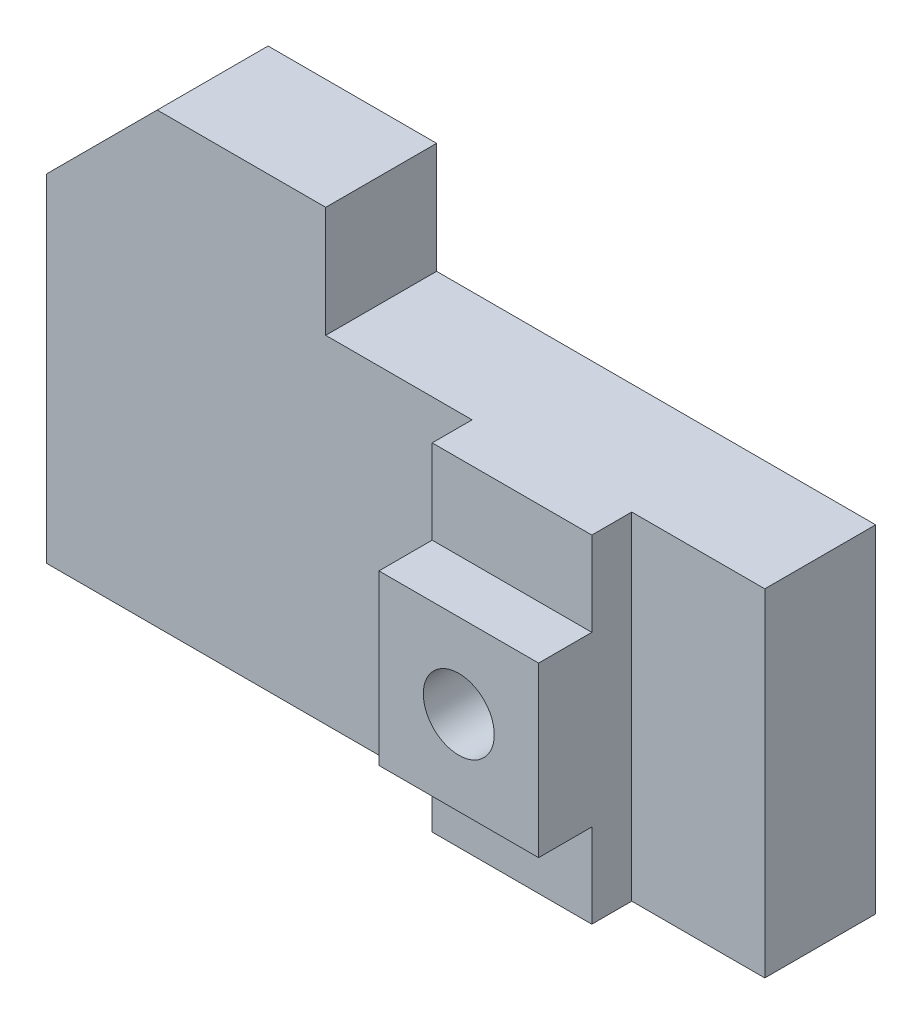
ISO-10303-21;
HEADER;
FILE_DESCRIPTION(('STEP AP214'),'2;1');
FILE_NAME('part.step','',(''),(''),'','','');
FILE_SCHEMA(('AUTOMOTIVE_DESIGN { 1 0 10303 214 1 1 1 1 }'));
ENDSEC;
DATA;
#1=APPLICATION_CONTEXT('core data for automotive mechanical design processes');
#2=APPLICATION_PROTOCOL_DEFINITION('international standard','automotive_design',2000,#1);
#3=PRODUCT_CONTEXT('',#1,'mechanical');
#4=PRODUCT('Part','Part','',(#3));
#5=PRODUCT_RELATED_PRODUCT_CATEGORY('part','',(#4));
#6=PRODUCT_DEFINITION_FORMATION('','',#4);
#7=PRODUCT_DEFINITION_CONTEXT('part definition',#1,'design');
#8=PRODUCT_DEFINITION('design','',#6,#7);
#9=PRODUCT_DEFINITION_SHAPE('','',#8);
#10=(LENGTH_UNIT() NAMED_UNIT(*) SI_UNIT(.MILLI.,.METRE.));
#11=(NAMED_UNIT(*) PLANE_ANGLE_UNIT() SI_UNIT($,.RADIAN.));
#12=(NAMED_UNIT(*) SI_UNIT($,.STERADIAN.) SOLID_ANGLE_UNIT());
#13=UNCERTAINTY_MEASURE_WITH_UNIT(LENGTH_MEASURE(1.E-05),#10,'distance_accuracy_value','');
#14=(GEOMETRIC_REPRESENTATION_CONTEXT(3) GLOBAL_UNCERTAINTY_ASSIGNED_CONTEXT((#13)) GLOBAL_UNIT_ASSIGNED_CONTEXT((#10,
#11,#12)) REPRESENTATION_CONTEXT('',''));
#15=CARTESIAN_POINT('',(0.,0.,0.));
#16=DIRECTION('',(0.,0.,1.));
#17=DIRECTION('',(1.,0.,0.));
#18=AXIS2_PLACEMENT_3D('',#15,#16,#17);
#19=CARTESIAN_POINT('',(0.,0.,34.));
#20=DIRECTION('',(0.,0.,-1.));
#21=DIRECTION('',(-1.,0.,0.));
#22=AXIS2_PLACEMENT_3D('',#19,#20,#21);
#23=PLANE('',#22);
#24=DIRECTION('',(-1.,0.,0.));
#25=VECTOR('',#24,1.);
#26=CARTESIAN_POINT('',(96.,57.,34.));
#27=LINE('',#26,#25);
#28=CARTESIAN_POINT('',(132.,57.,34.));
#29=VERTEX_POINT('',#28);
#30=CARTESIAN_POINT('',(96.,57.,34.));
#31=VERTEX_POINT('',#30);
#32=EDGE_CURVE('E173',#29,#31,#27,.T.);
#33=ORIENTED_EDGE('',*,*,#32,.F.);
#34=DIRECTION('',(0.,1.,0.));
#35=VECTOR('',#34,1.);
#36=CARTESIAN_POINT('',(132.,76.,34.));
#37=LINE('',#36,#35);
#38=CARTESIAN_POINT('',(132.,76.,34.));
#39=VERTEX_POINT('',#38);
#40=EDGE_CURVE('E187',#29,#39,#37,.T.);
#41=ORIENTED_EDGE('',*,*,#40,.T.);
#42=DIRECTION('',(-1.,0.,0.));
#43=VECTOR('',#42,1.);
#44=CARTESIAN_POINT('',(96.,76.,34.));
#45=LINE('',#44,#43);
#46=CARTESIAN_POINT('',(96.,76.,34.));
#47=VERTEX_POINT('',#46);
#48=EDGE_CURVE('E195',#39,#47,#45,.T.);
#49=ORIENTED_EDGE('',*,*,#48,.T.);
#50=DIRECTION('',(0.,-1.,0.));
#51=VECTOR('',#50,1.);
#52=CARTESIAN_POINT('',(96.,0.,34.));
#53=LINE('',#52,#51);
#54=EDGE_CURVE('E68',#47,#31,#53,.T.);
#55=ORIENTED_EDGE('',*,*,#54,.T.);
#56=EDGE_LOOP('',(#33,#41,#49,#55));
#57=FACE_BOUND('',#56,.T.);
#58=ADVANCED_FACE('F44',(#57),#23,.F.);
#59=DIRECTION('',(1.,0.,0.));
#60=VECTOR('',#59,1.);
#61=CARTESIAN_POINT('',(132.,19.,34.));
#62=LINE('',#61,#60);
#63=CARTESIAN_POINT('',(96.,19.,34.));
#64=VERTEX_POINT('',#63);
#65=CARTESIAN_POINT('',(132.,19.,34.));
#66=VERTEX_POINT('',#65);
#67=EDGE_CURVE('E58',#64,#66,#62,.T.);
#68=ORIENTED_EDGE('',*,*,#67,.F.);
#69=CARTESIAN_POINT('',(96.,0.,34.));
#70=VERTEX_POINT('',#69);
#71=EDGE_CURVE('E176',#64,#70,#53,.T.);
#72=ORIENTED_EDGE('',*,*,#71,.T.);
#73=DIRECTION('',(1.,0.,0.));
#74=VECTOR('',#73,1.);
#75=CARTESIAN_POINT('',(132.,0.,34.));
#76=LINE('',#75,#74);
#77=CARTESIAN_POINT('',(132.,0.,34.));
#78=VERTEX_POINT('',#77);
#79=EDGE_CURVE('E188',#70,#78,#76,.T.);
#80=ORIENTED_EDGE('',*,*,#79,.T.);
#81=EDGE_CURVE('E189',#78,#66,#37,.T.);
#82=ORIENTED_EDGE('',*,*,#81,.T.);
#83=EDGE_LOOP('',(#68,#72,#80,#82));
#84=FACE_BOUND('',#83,.T.);
#85=ADVANCED_FACE('F286',(#84),#23,.F.);
#86=CARTESIAN_POINT('',(0.,0.,25.));
#87=DIRECTION('',(0.,0.,-1.));
#88=DIRECTION('',(-1.,0.,0.));
#89=AXIS2_PLACEMENT_3D('',#86,#87,#88);
#90=PLANE('',#89);
#91=DIRECTION('',(0.,-1.,0.));
#92=VECTOR('',#91,1.);
#93=CARTESIAN_POINT('',(96.,0.,25.));
#94=LINE('',#93,#92);
#95=CARTESIAN_POINT('',(96.,76.,25.));
#96=VERTEX_POINT('',#95);
#97=CARTESIAN_POINT('',(96.,0.,25.));
#98=VERTEX_POINT('',#97);
#99=EDGE_CURVE('E179',#96,#98,#94,.T.);
#100=ORIENTED_EDGE('',*,*,#99,.F.);
#101=DIRECTION('',(-1.,0.,0.));
#102=VECTOR('',#101,1.);
#103=CARTESIAN_POINT('',(162.,76.,25.));
#104=LINE('',#103,#102);
#105=CARTESIAN_POINT('',(63.,76.,25.));
#106=VERTEX_POINT('',#105);
#107=EDGE_CURVE('E245',#96,#106,#104,.T.);
#108=ORIENTED_EDGE('',*,*,#107,.T.);
#109=DIRECTION('',(0.,1.,0.));
#110=VECTOR('',#109,1.);
#111=CARTESIAN_POINT('',(63.,76.,25.));
#112=LINE('',#111,#110);
#113=CARTESIAN_POINT('',(63.,101.,25.));
#114=VERTEX_POINT('',#113);
#115=EDGE_CURVE('E208',#106,#114,#112,.T.);
#116=ORIENTED_EDGE('',*,*,#115,.T.);
#117=DIRECTION('',(-1.,0.,0.));
#118=VECTOR('',#117,1.);
#119=CARTESIAN_POINT('',(63.,101.,25.));
#120=LINE('',#119,#118);
#121=CARTESIAN_POINT('',(25.,101.,25.));
#122=VERTEX_POINT('',#121);
#123=EDGE_CURVE('E222',#114,#122,#120,.T.);
#124=ORIENTED_EDGE('',*,*,#123,.T.);
#125=DIRECTION('',(-0.707106781186547,-0.707106781186548,0.));
#126=VECTOR('',#125,1.);
#127=CARTESIAN_POINT('',(25.,101.,25.));
#128=LINE('',#127,#126);
#129=CARTESIAN_POINT('',(0.,76.,25.));
#130=VERTEX_POINT('',#129);
#131=EDGE_CURVE('E213',#122,#130,#128,.T.);
#132=ORIENTED_EDGE('',*,*,#131,.T.);
#133=DIRECTION('',(0.,-1.,0.));
#134=VECTOR('',#133,1.);
#135=CARTESIAN_POINT('',(0.,0.,25.));
#136=LINE('',#135,#134);
#137=CARTESIAN_POINT('',(0.,0.,25.));
#138=VERTEX_POINT('',#137);
#139=EDGE_CURVE('E233',#130,#138,#136,.T.);
#140=ORIENTED_EDGE('',*,*,#139,.T.);
#141=DIRECTION('',(1.,0.,0.));
#142=VECTOR('',#141,1.);
#143=CARTESIAN_POINT('',(0.,0.,25.));
#144=LINE('',#143,#142);
#145=EDGE_CURVE('E236',#138,#98,#144,.T.);
#146=ORIENTED_EDGE('',*,*,#145,.T.);
#147=EDGE_LOOP('',(#100,#108,#116,#124,#132,#140,#146));
#148=FACE_BOUND('',#147,.T.);
#149=ADVANCED_FACE('F287',(#148),#90,.F.);
#150=DIRECTION('',(0.,1.,0.));
#151=VECTOR('',#150,1.);
#152=CARTESIAN_POINT('',(132.,76.,25.));
#153=LINE('',#152,#151);
#154=CARTESIAN_POINT('',(132.,0.,25.));
#155=VERTEX_POINT('',#154);
#156=CARTESIAN_POINT('',(132.,76.,25.));
#157=VERTEX_POINT('',#156);
#158=EDGE_CURVE('E180',#155,#157,#153,.T.);
#159=ORIENTED_EDGE('',*,*,#158,.F.);
#160=CARTESIAN_POINT('',(162.,0.,25.));
#161=VERTEX_POINT('',#160);
#162=EDGE_CURVE('E237',#155,#161,#144,.T.);
#163=ORIENTED_EDGE('',*,*,#162,.T.);
#164=DIRECTION('',(0.,1.,0.));
#165=VECTOR('',#164,1.);
#166=CARTESIAN_POINT('',(162.,0.,25.));
#167=LINE('',#166,#165);
#168=CARTESIAN_POINT('',(162.,76.,25.));
#169=VERTEX_POINT('',#168);
#170=EDGE_CURVE('E238',#161,#169,#167,.T.);
#171=ORIENTED_EDGE('',*,*,#170,.T.);
#172=EDGE_CURVE('E241',#169,#157,#104,.T.);
#173=ORIENTED_EDGE('',*,*,#172,.T.);
#174=EDGE_LOOP('',(#159,#163,#171,#173));
#175=FACE_BOUND('',#174,.T.);
#176=ADVANCED_FACE('F278',(#175),#90,.F.);
#177=CARTESIAN_POINT('',(0.,0.,25.));
#178=DIRECTION('',(0.,1.,0.));
#179=DIRECTION('',(0.,0.,1.));
#180=AXIS2_PLACEMENT_3D('',#177,#178,#179);
#181=PLANE('',#180);
#182=DIRECTION('',(1.,0.,0.));
#183=VECTOR('',#182,1.);
#184=CARTESIAN_POINT('',(0.,0.,0.));
#185=LINE('',#184,#183);
#186=CARTESIAN_POINT('',(0.,0.,0.));
#187=VERTEX_POINT('',#186);
#188=CARTESIAN_POINT('',(162.,0.,0.));
#189=VERTEX_POINT('',#188);
#190=EDGE_CURVE('E226',#187,#189,#185,.T.);
#191=ORIENTED_EDGE('',*,*,#190,.T.);
#192=DIRECTION('',(0.,0.,-1.));
#193=VECTOR('',#192,1.);
#194=CARTESIAN_POINT('',(162.,0.,25.));
#195=LINE('',#194,#193);
#196=EDGE_CURVE('E52',#161,#189,#195,.T.);
#197=ORIENTED_EDGE('',*,*,#196,.F.);
#198=ORIENTED_EDGE('',*,*,#162,.F.);
#199=DIRECTION('',(0.,0.,-1.));
#200=VECTOR('',#199,1.);
#201=CARTESIAN_POINT('',(132.,0.,34.));
#202=LINE('',#201,#200);
#203=EDGE_CURVE('E202',#78,#155,#202,.T.);
#204=ORIENTED_EDGE('',*,*,#203,.F.);
#205=ORIENTED_EDGE('',*,*,#79,.F.);
#206=DIRECTION('',(0.,0.,-1.));
#207=VECTOR('',#206,1.);
#208=CARTESIAN_POINT('',(96.,0.,34.));
#209=LINE('',#208,#207);
#210=EDGE_CURVE('E192',#70,#98,#209,.T.);
#211=ORIENTED_EDGE('',*,*,#210,.T.);
#212=ORIENTED_EDGE('',*,*,#145,.F.);
#213=DIRECTION('',(0.,0.,-1.));
#214=VECTOR('',#213,1.);
#215=CARTESIAN_POINT('',(0.,0.,25.));
#216=LINE('',#215,#214);
#217=EDGE_CURVE('E11',#138,#187,#216,.T.);
#218=ORIENTED_EDGE('',*,*,#217,.T.);
#219=EDGE_LOOP('',(#191,#197,#198,#204,#205,#211,#212,#218));
#220=FACE_BOUND('',#219,.T.);
#221=ADVANCED_FACE('F50',(#220),#181,.F.);
#222=CARTESIAN_POINT('',(162.,0.,25.));
#223=DIRECTION('',(-1.,0.,0.));
#224=DIRECTION('',(0.,0.,1.));
#225=AXIS2_PLACEMENT_3D('',#222,#223,#224);
#226=PLANE('',#225);
#227=DIRECTION('',(0.,1.,0.));
#228=VECTOR('',#227,1.);
#229=CARTESIAN_POINT('',(162.,0.,0.));
#230=LINE('',#229,#228);
#231=CARTESIAN_POINT('',(162.,76.,0.));
#232=VERTEX_POINT('',#231);
#233=EDGE_CURVE('E250',#189,#232,#230,.T.);
#234=ORIENTED_EDGE('',*,*,#233,.T.);
#235=DIRECTION('',(0.,0.,-1.));
#236=VECTOR('',#235,1.);
#237=CARTESIAN_POINT('',(162.,76.,25.));
#238=LINE('',#237,#236);
#239=EDGE_CURVE('E258',#169,#232,#238,.T.);
#240=ORIENTED_EDGE('',*,*,#239,.F.);
#241=ORIENTED_EDGE('',*,*,#170,.F.);
#242=ORIENTED_EDGE('',*,*,#196,.T.);
#243=EDGE_LOOP('',(#234,#240,#241,#242));
#244=FACE_BOUND('',#243,.T.);
#245=ADVANCED_FACE('F263',(#244),#226,.F.);
#246=CARTESIAN_POINT('',(0.,76.,25.));
#247=DIRECTION('',(0.,-1.,0.));
#248=DIRECTION('',(0.,0.,-1.));
#249=AXIS2_PLACEMENT_3D('',#246,#247,#248);
#250=PLANE('',#249);
#251=DIRECTION('',(-1.,0.,0.));
#252=VECTOR('',#251,1.);
#253=CARTESIAN_POINT('',(0.,76.,0.));
#254=LINE('',#253,#252);
#255=CARTESIAN_POINT('',(63.,76.,0.));
#256=VERTEX_POINT('',#255);
#257=EDGE_CURVE('E249',#232,#256,#254,.T.);
#258=ORIENTED_EDGE('',*,*,#257,.T.);
#259=DIRECTION('',(0.,0.,1.));
#260=VECTOR('',#259,1.);
#261=CARTESIAN_POINT('',(63.,76.,0.));
#262=LINE('',#261,#260);
#263=EDGE_CURVE('E217',#256,#106,#262,.T.);
#264=ORIENTED_EDGE('',*,*,#263,.T.);
#265=ORIENTED_EDGE('',*,*,#107,.F.);
#266=DIRECTION('',(0.,0.,-1.));
#267=VECTOR('',#266,1.);
#268=CARTESIAN_POINT('',(96.,76.,34.));
#269=LINE('',#268,#267);
#270=EDGE_CURVE('E200',#47,#96,#269,.T.);
#271=ORIENTED_EDGE('',*,*,#270,.F.);
#272=ORIENTED_EDGE('',*,*,#48,.F.);
#273=DIRECTION('',(0.,0.,-1.));
#274=VECTOR('',#273,1.);
#275=CARTESIAN_POINT('',(132.,76.,34.));
#276=LINE('',#275,#274);
#277=EDGE_CURVE('E205',#39,#157,#276,.T.);
#278=ORIENTED_EDGE('',*,*,#277,.T.);
#279=ORIENTED_EDGE('',*,*,#172,.F.);
#280=ORIENTED_EDGE('',*,*,#239,.T.);
#281=EDGE_LOOP('',(#258,#264,#265,#271,#272,#278,#279,#280));
#282=FACE_BOUND('',#281,.T.);
#283=ADVANCED_FACE('F273',(#282),#250,.F.);
#284=CARTESIAN_POINT('',(0.,51.,25.));
#285=DIRECTION('',(1.,0.,0.));
#286=DIRECTION('',(0.,0.,-1.));
#287=AXIS2_PLACEMENT_3D('',#284,#285,#286);
#288=PLANE('',#287);
#289=DIRECTION('',(0.,-1.,0.));
#290=VECTOR('',#289,1.);
#291=CARTESIAN_POINT('',(0.,51.,0.));
#292=LINE('',#291,#290);
#293=CARTESIAN_POINT('',(0.,76.,0.));
#294=VERTEX_POINT('',#293);
#295=EDGE_CURVE('E240',#294,#187,#292,.T.);
#296=ORIENTED_EDGE('',*,*,#295,.T.);
#297=ORIENTED_EDGE('',*,*,#217,.F.);
#298=ORIENTED_EDGE('',*,*,#139,.F.);
#299=DIRECTION('',(0.,0.,-1.));
#300=VECTOR('',#299,1.);
#301=CARTESIAN_POINT('',(0.,76.,25.));
#302=LINE('',#301,#300);
#303=EDGE_CURVE('E244',#130,#294,#302,.T.);
#304=ORIENTED_EDGE('',*,*,#303,.T.);
#305=EDGE_LOOP('',(#296,#297,#298,#304));
#306=FACE_BOUND('',#305,.T.);
#307=ADVANCED_FACE('F349',(#306),#288,.F.);
#308=CARTESIAN_POINT('',(0.,0.,0.));
#309=DIRECTION('',(0.,0.,-1.));
#310=DIRECTION('',(-1.,0.,0.));
#311=AXIS2_PLACEMENT_3D('',#308,#309,#310);
#312=PLANE('',#311);
#313=ORIENTED_EDGE('',*,*,#190,.F.);
#314=ORIENTED_EDGE('',*,*,#295,.F.);
#315=DIRECTION('',(-0.707106781186547,-0.707106781186548,0.));
#316=VECTOR('',#315,1.);
#317=CARTESIAN_POINT('',(25.,101.,0.));
#318=LINE('',#317,#316);
#319=CARTESIAN_POINT('',(25.,101.,0.));
#320=VERTEX_POINT('',#319);
#321=EDGE_CURVE('E216',#320,#294,#318,.T.);
#322=ORIENTED_EDGE('',*,*,#321,.F.);
#323=DIRECTION('',(-1.,0.,0.));
#324=VECTOR('',#323,1.);
#325=CARTESIAN_POINT('',(63.,101.,0.));
#326=LINE('',#325,#324);
#327=CARTESIAN_POINT('',(63.,101.,0.));
#328=VERTEX_POINT('',#327);
#329=EDGE_CURVE('E215',#328,#320,#326,.T.);
#330=ORIENTED_EDGE('',*,*,#329,.F.);
#331=DIRECTION('',(0.,1.,0.));
#332=VECTOR('',#331,1.);
#333=CARTESIAN_POINT('',(63.,76.,0.));
#334=LINE('',#333,#332);
#335=EDGE_CURVE('E207',#256,#328,#334,.T.);
#336=ORIENTED_EDGE('',*,*,#335,.F.);
#337=ORIENTED_EDGE('',*,*,#257,.F.);
#338=ORIENTED_EDGE('',*,*,#233,.F.);
#339=EDGE_LOOP('',(#313,#314,#322,#330,#336,#337,#338));
#340=FACE_BOUND('',#339,.T.);
#341=ADVANCED_FACE('F267',(#340),#312,.T.);
#342=CARTESIAN_POINT('',(25.,101.,0.));
#343=DIRECTION('',(-0.707106781186548,0.707106781186547,0.));
#344=DIRECTION('',(-0.707106781186547,-0.707106781186548,0.));
#345=AXIS2_PLACEMENT_3D('',#342,#343,#344);
#346=PLANE('',#345);
#347=ORIENTED_EDGE('',*,*,#131,.F.);
#348=DIRECTION('',(0.,0.,1.));
#349=VECTOR('',#348,1.);
#350=CARTESIAN_POINT('',(25.,101.,0.));
#351=LINE('',#350,#349);
#352=EDGE_CURVE('E228',#320,#122,#351,.T.);
#353=ORIENTED_EDGE('',*,*,#352,.F.);
#354=ORIENTED_EDGE('',*,*,#321,.T.);
#355=ORIENTED_EDGE('',*,*,#303,.F.);
#356=EDGE_LOOP('',(#347,#353,#354,#355));
#357=FACE_BOUND('',#356,.T.);
#358=ADVANCED_FACE('F331',(#357),#346,.T.);
#359=CARTESIAN_POINT('',(63.,101.,0.));
#360=DIRECTION('',(0.,1.,0.));
#361=DIRECTION('',(0.,0.,1.));
#362=AXIS2_PLACEMENT_3D('',#359,#360,#361);
#363=PLANE('',#362);
#364=ORIENTED_EDGE('',*,*,#123,.F.);
#365=DIRECTION('',(0.,0.,1.));
#366=VECTOR('',#365,1.);
#367=CARTESIAN_POINT('',(63.,101.,0.));
#368=LINE('',#367,#366);
#369=EDGE_CURVE('E227',#328,#114,#368,.T.);
#370=ORIENTED_EDGE('',*,*,#369,.F.);
#371=ORIENTED_EDGE('',*,*,#329,.T.);
#372=ORIENTED_EDGE('',*,*,#352,.T.);
#373=EDGE_LOOP('',(#364,#370,#371,#372));
#374=FACE_BOUND('',#373,.T.);
#375=ADVANCED_FACE('F340',(#374),#363,.T.);
#376=CARTESIAN_POINT('',(63.,76.,0.));
#377=DIRECTION('',(1.,0.,0.));
#378=DIRECTION('',(0.,0.,-1.));
#379=AXIS2_PLACEMENT_3D('',#376,#377,#378);
#380=PLANE('',#379);
#381=ORIENTED_EDGE('',*,*,#115,.F.);
#382=ORIENTED_EDGE('',*,*,#263,.F.);
#383=ORIENTED_EDGE('',*,*,#335,.T.);
#384=ORIENTED_EDGE('',*,*,#369,.T.);
#385=EDGE_LOOP('',(#381,#382,#383,#384));
#386=FACE_BOUND('',#385,.T.);
#387=ADVANCED_FACE('F334',(#386),#380,.T.);
#388=CARTESIAN_POINT('',(132.,76.,34.));
#389=DIRECTION('',(-1.,0.,0.));
#390=DIRECTION('',(0.,0.,1.));
#391=AXIS2_PLACEMENT_3D('',#388,#389,#390);
#392=PLANE('',#391);
#393=ORIENTED_EDGE('',*,*,#158,.T.);
#394=ORIENTED_EDGE('',*,*,#277,.F.);
#395=ORIENTED_EDGE('',*,*,#40,.F.);
#396=DIRECTION('',(0.,0.,-1.));
#397=VECTOR('',#396,1.);
#398=CARTESIAN_POINT('',(132.,57.,46.));
#399=LINE('',#398,#397);
#400=CARTESIAN_POINT('',(132.,57.,46.));
#401=VERTEX_POINT('',#400);
#402=EDGE_CURVE('E185',#401,#29,#399,.T.);
#403=ORIENTED_EDGE('',*,*,#402,.F.);
#404=DIRECTION('',(0.,1.,0.));
#405=VECTOR('',#404,1.);
#406=CARTESIAN_POINT('',(132.,57.,46.));
#407=LINE('',#406,#405);
#408=CARTESIAN_POINT('',(132.,19.,46.));
#409=VERTEX_POINT('',#408);
#410=EDGE_CURVE('E161',#409,#401,#407,.T.);
#411=ORIENTED_EDGE('',*,*,#410,.F.);
#412=DIRECTION('',(0.,0.,-1.));
#413=VECTOR('',#412,1.);
#414=CARTESIAN_POINT('',(132.,19.,46.));
#415=LINE('',#414,#413);
#416=EDGE_CURVE('E158',#409,#66,#415,.T.);
#417=ORIENTED_EDGE('',*,*,#416,.T.);
#418=ORIENTED_EDGE('',*,*,#81,.F.);
#419=ORIENTED_EDGE('',*,*,#203,.T.);
#420=EDGE_LOOP('',(#393,#394,#395,#403,#411,#417,#418,#419));
#421=FACE_BOUND('',#420,.T.);
#422=ADVANCED_FACE('F285',(#421),#392,.F.);
#423=CARTESIAN_POINT('',(96.,0.,34.));
#424=DIRECTION('',(1.,0.,0.));
#425=DIRECTION('',(0.,0.,-1.));
#426=AXIS2_PLACEMENT_3D('',#423,#424,#425);
#427=PLANE('',#426);
#428=ORIENTED_EDGE('',*,*,#99,.T.);
#429=ORIENTED_EDGE('',*,*,#210,.F.);
#430=ORIENTED_EDGE('',*,*,#71,.F.);
#431=DIRECTION('',(0.,0.,-1.));
#432=VECTOR('',#431,1.);
#433=CARTESIAN_POINT('',(96.,19.,46.));
#434=LINE('',#433,#432);
#435=CARTESIAN_POINT('',(96.,19.,46.));
#436=VERTEX_POINT('',#435);
#437=EDGE_CURVE('E156',#436,#64,#434,.T.);
#438=ORIENTED_EDGE('',*,*,#437,.F.);
#439=DIRECTION('',(0.,-1.,0.));
#440=VECTOR('',#439,1.);
#441=CARTESIAN_POINT('',(96.,19.,46.));
#442=LINE('',#441,#440);
#443=CARTESIAN_POINT('',(96.,57.,46.));
#444=VERTEX_POINT('',#443);
#445=EDGE_CURVE('E165',#444,#436,#442,.T.);
#446=ORIENTED_EDGE('',*,*,#445,.F.);
#447=DIRECTION('',(0.,0.,-1.));
#448=VECTOR('',#447,1.);
#449=CARTESIAN_POINT('',(96.,57.,46.));
#450=LINE('',#449,#448);
#451=EDGE_CURVE('E292',#444,#31,#450,.T.);
#452=ORIENTED_EDGE('',*,*,#451,.T.);
#453=ORIENTED_EDGE('',*,*,#54,.F.);
#454=ORIENTED_EDGE('',*,*,#270,.T.);
#455=EDGE_LOOP('',(#428,#429,#430,#438,#446,#452,#453,#454));
#456=FACE_BOUND('',#455,.T.);
#457=ADVANCED_FACE('F172',(#456),#427,.F.);
#458=CARTESIAN_POINT('',(132.,19.,46.));
#459=DIRECTION('',(0.,1.,0.));
#460=DIRECTION('',(0.,0.,1.));
#461=AXIS2_PLACEMENT_3D('',#458,#459,#460);
#462=PLANE('',#461);
#463=ORIENTED_EDGE('',*,*,#67,.T.);
#464=ORIENTED_EDGE('',*,*,#416,.F.);
#465=DIRECTION('',(1.,0.,0.));
#466=VECTOR('',#465,1.);
#467=CARTESIAN_POINT('',(132.,19.,46.));
#468=LINE('',#467,#466);
#469=EDGE_CURVE('E155',#436,#409,#468,.T.);
#470=ORIENTED_EDGE('',*,*,#469,.F.);
#471=ORIENTED_EDGE('',*,*,#437,.T.);
#472=EDGE_LOOP('',(#463,#464,#470,#471));
#473=FACE_BOUND('',#472,.T.);
#474=ADVANCED_FACE('F152',(#473),#462,.F.);
#475=CARTESIAN_POINT('',(96.,57.,46.));
#476=DIRECTION('',(0.,-1.,0.));
#477=DIRECTION('',(0.,0.,-1.));
#478=AXIS2_PLACEMENT_3D('',#475,#476,#477);
#479=PLANE('',#478);
#480=ORIENTED_EDGE('',*,*,#32,.T.);
#481=ORIENTED_EDGE('',*,*,#451,.F.);
#482=DIRECTION('',(-1.,0.,0.));
#483=VECTOR('',#482,1.);
#484=CARTESIAN_POINT('',(96.,57.,46.));
#485=LINE('',#484,#483);
#486=EDGE_CURVE('E170',#401,#444,#485,.T.);
#487=ORIENTED_EDGE('',*,*,#486,.F.);
#488=ORIENTED_EDGE('',*,*,#402,.T.);
#489=EDGE_LOOP('',(#480,#481,#487,#488));
#490=FACE_BOUND('',#489,.T.);
#491=ADVANCED_FACE('F316',(#490),#479,.F.);
#492=CARTESIAN_POINT('',(0.,0.,46.));
#493=DIRECTION('',(0.,0.,-1.));
#494=DIRECTION('',(-1.,0.,0.));
#495=AXIS2_PLACEMENT_3D('',#492,#493,#494);
#496=PLANE('',#495);
#497=CARTESIAN_POINT('',(114.,38.,46.));
#498=DIRECTION('',(0.,0.,1.));
#499=DIRECTION('',(1.,0.,0.));
#500=AXIS2_PLACEMENT_3D('',#497,#498,#499);
#501=CIRCLE('',#500,8.);
#502=CARTESIAN_POINT('',(122.,38.,46.));
#503=VERTEX_POINT('',#502);
#504=EDGE_CURVE('E301',#503,#503,#501,.T.);
#505=ORIENTED_EDGE('',*,*,#504,.F.);
#506=EDGE_LOOP('',(#505));
#507=FACE_BOUND('',#506,.T.);
#508=ORIENTED_EDGE('',*,*,#445,.T.);
#509=ORIENTED_EDGE('',*,*,#469,.T.);
#510=ORIENTED_EDGE('',*,*,#410,.T.);
#511=ORIENTED_EDGE('',*,*,#486,.T.);
#512=EDGE_LOOP('',(#508,#509,#510,#511));
#513=FACE_BOUND('',#512,.T.);
#514=ADVANCED_FACE('F164',(#507,#513),#496,.F.);
#515=CARTESIAN_POINT('',(114.,38.,26.));
#516=DIRECTION('',(0.,0.,1.));
#517=DIRECTION('',(1.,0.,0.));
#518=AXIS2_PLACEMENT_3D('',#515,#516,#517);
#519=CYLINDRICAL_SURFACE('',#518,8.);
#520=CARTESIAN_POINT('',(114.,38.,26.));
#521=DIRECTION('',(0.,0.,1.));
#522=DIRECTION('',(1.,0.,0.));
#523=AXIS2_PLACEMENT_3D('',#520,#521,#522);
#524=CIRCLE('',#523,8.);
#525=CARTESIAN_POINT('',(122.,38.,26.));
#526=VERTEX_POINT('',#525);
#527=EDGE_CURVE('E296',#526,#526,#524,.T.);
#528=ORIENTED_EDGE('',*,*,#527,.F.);
#529=EDGE_LOOP('',(#528));
#530=FACE_BOUND('',#529,.T.);
#531=ORIENTED_EDGE('',*,*,#504,.T.);
#532=EDGE_LOOP('',(#531));
#533=FACE_BOUND('',#532,.T.);
#534=ADVANCED_FACE('F310',(#530,#533),#519,.F.);
#535=CARTESIAN_POINT('',(114.,38.,26.));
#536=DIRECTION('',(0.,0.,1.));
#537=DIRECTION('',(1.,0.,0.));
#538=AXIS2_PLACEMENT_3D('',#535,#536,#537);
#539=PLANE('',#538);
#540=ORIENTED_EDGE('',*,*,#527,.T.);
#541=EDGE_LOOP('',(#540));
#542=FACE_BOUND('',#541,.T.);
#543=ADVANCED_FACE('F307',(#542),#539,.T.);
#544=CLOSED_SHELL('',(#58,#85,#149,#176,#221,#245,#283,#307,#341,#358,#375,#387,#422,#457,#474,
#491,#514,#534,#543));
#545=MANIFOLD_SOLID_BREP('B2',#544);
#546=ADVANCED_BREP_SHAPE_REPRESENTATION('',(#18,#545),#14);
#547=SHAPE_DEFINITION_REPRESENTATION(#9,#546);
ENDSEC;
END-ISO-10303-21;
